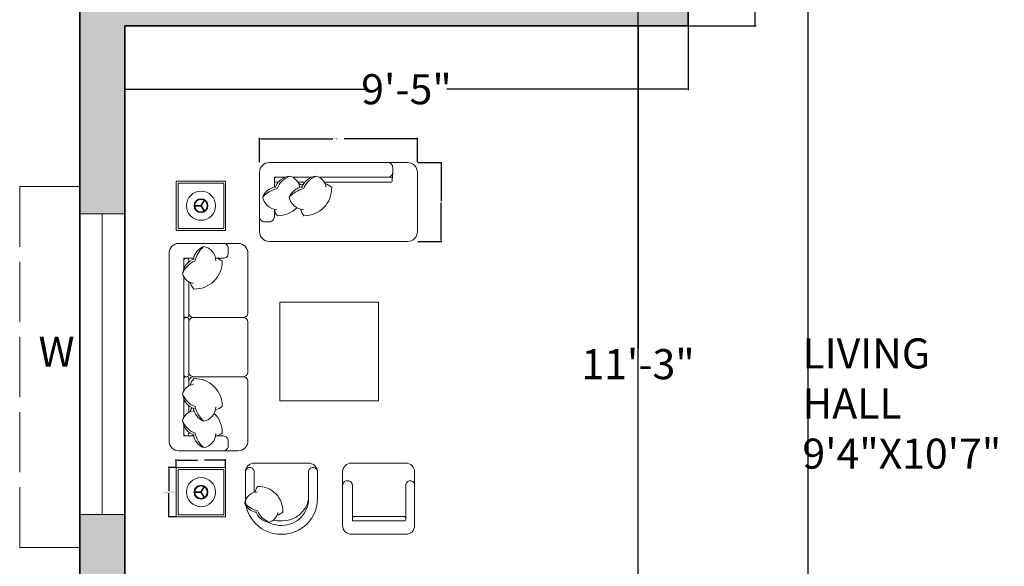
# Model space of a CAD drawing. Units: inches. Extents: x -5 to 482, y -460 to 66.
# Tile 13 of 31: x 21 to 218, y -252 to -143. Entities that reach past the tile are written whole.
import ezdxf

# ---------------------------------------------------------------- set-up
doc = ezdxf.new("R2010")
doc.units = ezdxf.units.IN
doc.header["$MEASUREMENT"] = 0
doc.linetypes.add('ACAD_ISO02W100', pattern=[15, 12, -3])
for name, color, linetype, lineweight in [('A-ANNO-DIMS', 2, 'Continuous', 18), ('A-ANNO-TEXT', 7, 'Continuous', 18), ('A-AREA-IDEN', 7, 'Continuous', 18), ('A-FURN', 8, 'Continuous', 18), ('A-GLAZ', 4, 'Continuous', 18), ('A-GLAZ-OVHD', 4, 'ACAD_ISO02W100', 13), ('A-WALL', 7, 'Continuous', 35), ('A-WALL-PATT', 152, 'Continuous', 13)]:
    doc.layers.add(name, color=color, linetype=linetype, lineweight=lineweight)
doc.styles.get("Standard").update_dxf_attribs({"font": 'arial.ttf'})
doc.dimstyles.get("Standard").update_dxf_attribs({"dimtxt": 0.18, "dimasz": 0.18, "dimexe": 0.18, "dimexo": 0.0625, "dimgap": 0.09, "dimtad": 0, "dimtih": 1, "dimtoh": 1, "dimdec": 0, "dimzin": 0, "dimdsep": 46, "dimlunit": 3, "dimtxsty": 'Standard', "dimcen": 0.09, "dimadec": 0, "dimazin": 0, "dimtfac": 1, "dimtdec": 0, "dimtofl": 0, "dimtmove": 0, "dimatfit": 3, "dimfxl": 1, "dimtolj": 1, "dimtzin": 0, "dimarcsym": 0})

# ---------------------------------------------------------------- blocks, each defined once
blk = doc.blocks.new('DAY BED1')
at = {"color": 0}
blk.add_line((0.3, 0.25), (0.225, 0.2549), dxfattribs=at)
blk.add_lwpolyline([(-0.3, 0, -0.414214), (-0.4, 0.1), (-0.4, 0.1, 0.317837), (-0.4, 0.1, -0.414214), (-0.4, 0.1), (-0.4, 0.1, 1.186185), (-0.4, 0.1, -0.414214), (-0.4, 0.1), (-0.4, 1.5, -0.414214), (-0.3, 1.6), (0.3, 1.6, -0.414214), (0.4, 1.5), (0.4, 0.1, -0.414214), (0.3, 0)], format="xyb", close=True, dxfattribs=at)
for points in [[(-0.0725, 1.45), (-0.15, 1.45, -0.414214), (-0.2, 1.5), (-0.2, 1.55, -0.414214), (-0.15, 1.6)], [(-0.0756, 1.4249, -0.356772), (0.0505, 1.5682, -0.249542), (0.1543, 1.4384, 9.61688)], [(0.0505, 1.5682, -0.14773), (0.1364, 1.422, -0.213343), (0.2624, 1.2931, -0.178662)], [(-0.0725, 1.4501, 0.165541), (-0.1386, 1.4192, 0.200231), (-0.0581, 1.2207, 0.121523)], [(0.1433, 1.4422, -0.306663), (0.2624, 1.2931, -0.30633), (0.1536, 1.1957, 0.872847)], [(0.25, 1.3448), (0.25, 1.45), (0.1517, 1.45, -0.414214)], [(0.2, 1.4118), (0.2, 1.43, -0.414214), (0.22, 1.45), (0.23, 1.45, -0.414214), (0.25, 1.43)], [(0.25, 1.43), (0.25, 1.3448, -0.414214)], [(-0.0756, 1.1556, -0.356772), (0.0505, 1.2988, -0.249542), (0.1543, 1.169, 9.61688)], [(0.0505, 1.2988, -0.14773), (0.1364, 1.1527, -0.213343), (0.2624, 1.0238, -0.178662)], [(0.1678, 1.1631, 0.071865), (0.1873, 1.205, -7.115464)], [(0.2, 1.1425), (0.2, 1.2113, -0.414214)], [(0.25, 1.2616), (0.25, 1.0755, -0.414214)], [(-0.0725, 1.1808, 0.165541), (-0.1386, 1.1498, 0.425989), (0.1479, 0.869, 0.121523), (0.1873, 0.9357, -7.115464)], [(0.1433, 1.1729, -0.306663), (0.2624, 1.0238, -0.30633), (0.1536, 0.9263, 0.872847)], [(0.25, 0.9923), (0.25, 0.2749, -0.414214), (0.23, 0.2549), (0.22, 0.2549, -0.414214), (0.2, 0.2749), (0.2, 0.9419, -0.414214)], [(0.25, 0.3775), (0.25, 0.3, 0.414214), (0.3, 0.25), (0.35, 0.25, 0.414214), (0.4, 0.3)]]:
    blk.add_lwpolyline(points, format="xyb", dxfattribs=at)
for points in [[(0.25, 1.0755), (0.25, 1.2616)], [(0.25, 0.3775), (0.25, 0.9923)]]:
    blk.add_lwpolyline(points, dxfattribs=at)
blk = doc.blocks.new('*D8')
at = {"layer": 'A-ANNO-DIMS', "color": 0, "lineweight": -2, "transparency": 16777216}
for p, q in [((154.44, 4.15), (167.95, 4.15)), ((167.77, 3.97), (167.77, -66.95)), ((167.77, -144.17), (167.77, -73.25)), ((154.44, -144.35), (167.95, -144.35))]:
    blk.add_line(p, q, dxfattribs=at)
at = {"layer": 'A-ANNO-DIMS', "color": 0, "transparency": 16777216}
for points in [[(167.74, 3.97), (167.8, 3.97), (167.77, 4.15)], [(167.74, -144.17), (167.8, -144.17), (167.77, -144.35)]]:
    blk.add_solid(points, dxfattribs=at)
at = {"layer": 'Defpoints', "color": 0, "transparency": 16777216}
for p in [(154.38, 4.15), (167.77, 4.15), (154.38, -144.35)]:
    blk.add_point(p, dxfattribs=at)
at = {"layer": 'A-ANNO-DIMS', "color": 0, "transparency": 16777216, "insert": (167.77, -70.1), "char_height": 6, "attachment_point": 5}
blk.add_mtext('\\A1;12\'-5"', dxfattribs=at)
blk = doc.blocks.new('*D18')
at = {"layer": 'A-ANNO-DIMS', "color": 0, "lineweight": -2, "transparency": 16777216}
for p, q in [((144.38, -144.53), (144.38, -208.69)), ((144.44, -144.35), (144.56, -144.35)), ((144.38, -279.17), (144.38, -215)), ((144.44, -279.35), (144.56, -279.35))]:
    blk.add_line(p, q, dxfattribs=at)
at = {"layer": 'A-ANNO-DIMS', "color": 0, "transparency": 16777216}
for points in [[(144.35, -144.53), (144.41, -144.53), (144.38, -144.35)], [(144.35, -279.17), (144.41, -279.17), (144.38, -279.35)]]:
    blk.add_solid(points, dxfattribs=at)
at = {"layer": 'Defpoints', "color": 0, "transparency": 16777216}
for p in [(144.38, -144.35), (144.38, -144.35), (144.38, -279.35)]:
    blk.add_point(p, dxfattribs=at)
at = {"layer": 'A-ANNO-DIMS', "color": 0, "transparency": 16777216, "insert": (144.38, -211.85), "char_height": 6, "attachment_point": 5}
blk.add_mtext('\\A1;11\'-3"', dxfattribs=at)
blk = doc.blocks.new('*D19')
at = {"layer": 'A-ANNO-DIMS', "color": 0, "lineweight": -2, "transparency": 16777216}
for p, q in [((41.88, -144.41), (41.88, -157.16)), ((154.38, -144.41), (154.38, -157.16)), ((42.06, -156.98), (90.06, -156.98)), ((154.2, -156.98), (106.19, -156.98))]:
    blk.add_line(p, q, dxfattribs=at)
at = {"layer": 'A-ANNO-DIMS', "color": 0, "transparency": 16777216}
for points in [[(42.06, -156.95), (42.06, -157.01), (41.88, -156.98)], [(154.2, -156.95), (154.2, -157.01), (154.38, -156.98)]]:
    blk.add_solid(points, dxfattribs=at)
at = {"layer": 'Defpoints', "color": 0, "transparency": 16777216}
for p in [(41.88, -144.35), (154.38, -144.35), (41.88, -156.98)]:
    blk.add_point(p, dxfattribs=at)
at = {"layer": 'A-ANNO-DIMS', "color": 0, "transparency": 16777216, "insert": (98.13, -156.98), "char_height": 6, "attachment_point": 5}
blk.add_mtext('\\A1;9\'-5"', dxfattribs=at)
blk = doc.blocks.new('WIN-GLAZ-60IN')
for p, q in [((0, 9), (60, 9)), ((0, 4.5), (60, 4.5)), ((60, 0), (0, 0))]:
    blk.add_line(p, q)
blk = doc.blocks.new('WIN-SHADE-72IN')
for p, q in [((0, 12), (72, 12)), ((0, 12), (0, 0)), ((72, 12), (72, 0))]:
    blk.add_line(p, q)
blk = doc.blocks.new('END-TABLE-WITH-LAMP')
for p, q in [((4.87, 4.96), (5.57, 6.16)), ((4.98, 4.9), (5.68, 6.1)), ((4.93, 4.99), (3.54, 4.99)), ((4.93, 4.86), (3.54, 4.86)), ((4.87, 4.9), (5.57, 3.69)), ((4.98, 4.96), (5.68, 3.75))]:
    blk.add_line(p, q)
at = {"ltscale": 0.03}
blk.add_lwpolyline([(9.85, 9.85), (9.85, 0), (0, 0), (0, 9.85)], close=True, dxfattribs=at)
blk.add_lwpolyline([(9.46, 0.39), (9.46, 9.46), (0.39, 9.46), (0.39, 0.39)], close=True)
for radius in [2.91, 1.39, 1.25]:
    blk.add_circle((4.93, 4.93), radius)
blk = doc.blocks.new('*D53')
at = {"layer": 'A-ANNO-DIMS', "color": 0, "lineweight": -2, "transparency": 16777216}
for p, q in [((52.1, -232.46), (50.5, -232.46)), ((50.68, -232.64), (50.68, -237.2)), ((50.68, -242.13), (50.68, -237.56)), ((52.1, -242.31), (50.5, -242.31))]:
    blk.add_line(p, q, dxfattribs=at)
at = {"layer": 'A-ANNO-DIMS', "color": 0, "transparency": 16777216}
for points in [[(50.65, -232.64), (50.71, -232.64), (50.68, -232.46)], [(50.65, -242.13), (50.71, -242.13), (50.68, -242.31)]]:
    blk.add_solid(points, dxfattribs=at)
at = {"layer": 'Defpoints', "color": 0, "transparency": 16777216}
for p in [(50.68, -232.46), (52.16, -232.46), (52.16, -242.31)]:
    blk.add_point(p, dxfattribs=at)
at = {"layer": 'A-ANNO-DIMS', "color": 0, "transparency": 16777216, "insert": (50.68, -237.38), "char_height": 0.18, "attachment_point": 5}
blk.add_mtext('\\A1;END TABLE 0\'-10" TYP.', dxfattribs=at)
blk = doc.blocks.new('*D54')
at = {"layer": 'A-ANNO-DIMS', "color": 0, "lineweight": -2, "transparency": 16777216}
for p, q in [((52.16, -232.39), (52.16, -230.8)), ((52.34, -230.98), (56.38, -230.98)), ((61.83, -230.98), (57.79, -230.98)), ((62.01, -232.39), (62.01, -230.8))]:
    blk.add_line(p, q, dxfattribs=at)
at = {"layer": 'A-ANNO-DIMS', "color": 0, "transparency": 16777216}
for points in [[(52.34, -230.95), (52.34, -231.01), (52.16, -230.98)], [(61.83, -230.95), (61.83, -231.01), (62.01, -230.98)]]:
    blk.add_solid(points, dxfattribs=at)
at = {"layer": 'Defpoints', "color": 0, "transparency": 16777216}
for p in [(62.01, -230.98), (52.16, -232.46), (62.01, -232.46)]:
    blk.add_point(p, dxfattribs=at)
at = {"layer": 'A-ANNO-DIMS', "color": 0, "transparency": 16777216, "insert": (57.09, -230.98), "char_height": 0.18, "attachment_point": 5}
blk.add_mtext('\\A1;0\'-10" TYP.', dxfattribs=at)
blk = doc.blocks.new('*D65')
at = {"layer": 'A-ANNO-DIMS', "color": 0, "lineweight": -2, "transparency": 16777216}
for p, q in [((68.78, -171.55), (68.78, -166.7)), ((68.96, -166.88), (83.42, -166.88)), ((100.13, -166.88), (85.66, -166.88)), ((100.31, -171.55), (100.31, -166.7))]:
    blk.add_line(p, q, dxfattribs=at)
at = {"layer": 'A-ANNO-DIMS', "color": 0, "transparency": 16777216}
for points in [[(68.96, -166.85), (68.96, -166.91), (68.78, -166.88)], [(100.13, -166.85), (100.13, -166.91), (100.31, -166.88)]]:
    blk.add_solid(points, dxfattribs=at)
at = {"layer": 'Defpoints', "color": 0, "transparency": 16777216}
for p in [(68.78, -166.88), (68.78, -171.61), (100.31, -171.61)]:
    blk.add_point(p, dxfattribs=at)
at = {"layer": 'A-ANNO-DIMS', "color": 0, "transparency": 16777216, "insert": (84.54, -166.88), "char_height": 0.18, "attachment_point": 5}
blk.add_mtext('\\A1;DAY BED 2\'-7 1/2"', dxfattribs=at)
blk = doc.blocks.new('*D66')
at = {"layer": 'A-ANNO-DIMS', "color": 0, "lineweight": -2, "transparency": 16777216}
for p, q in [((100.37, -171.61), (105.22, -171.61)), ((105.04, -171.79), (105.04, -179.31)), ((105.04, -187.19), (105.04, -179.67)), ((100.37, -187.37), (105.22, -187.37))]:
    blk.add_line(p, q, dxfattribs=at)
at = {"layer": 'A-ANNO-DIMS', "color": 0, "transparency": 16777216}
for points in [[(105.01, -171.79), (105.07, -171.79), (105.04, -171.61)], [(105.01, -187.19), (105.07, -187.19), (105.04, -187.37)]]:
    blk.add_solid(points, dxfattribs=at)
at = {"layer": 'Defpoints', "color": 0, "transparency": 16777216}
for p in [(100.31, -171.61), (105.04, -171.61), (100.31, -187.37)]:
    blk.add_point(p, dxfattribs=at)
at = {"layer": 'A-ANNO-DIMS', "color": 0, "transparency": 16777216, "insert": (105.04, -179.49), "char_height": 0.18, "attachment_point": 5}
blk.add_mtext('\\A1;1\'-4"', dxfattribs=at)
blk = doc.blocks.new('*D73')
at = {"layer": 'A-ANNO-DIMS', "color": 0, "lineweight": -2, "transparency": 16777216}
for p, q in [((144.38, -295.8), (144.38, 50.93)), ((144.56, 50.75), (160.98, 50.75)), ((178.2, 50.75), (161.78, 50.75)), ((178.38, -295.8), (178.38, 50.93))]:
    blk.add_line(p, q, dxfattribs=at)
at = {"layer": 'A-ANNO-DIMS', "color": 0, "transparency": 16777216}
for points in [[(144.56, 50.78), (144.56, 50.72), (144.38, 50.75)], [(178.2, 50.78), (178.2, 50.72), (178.38, 50.75)]]:
    blk.add_solid(points, dxfattribs=at)
at = {"layer": 'Defpoints', "color": 0, "transparency": 16777216}
for p in [(178.38, 50.75), (144.38, -295.86), (178.38, -295.86)]:
    blk.add_point(p, dxfattribs=at)
at = {"layer": 'A-ANNO-DIMS', "color": 0, "transparency": 16777216, "insert": (161.38, 50.75), "char_height": 0.18, "attachment_point": 5}
blk.add_mtext('\\A1;2\'-10"', dxfattribs=at)

msp = doc.modelspace()

# ---------------------------------------------------------------- hatches: boundary and pattern name
at = {"layer": 'A-WALL-PATT'}
h = msp.add_hatch(color=256, dxfattribs=at)
h.dxf.hatch_style = 1
h.paths.add_polyline_path([(149.38, -412.85), (144.38, -412.85), (144.38, -283.85), (144.38, -279.35), (133.88, -279.35), (133.88, -283.85), (139.88, -283.85), (139.88, -412.85), (133.51, -412.85), (133.51, -413.92), (102.65, -413.92), (102.65, -421.02), (133.51, -421.02), (133.51, -421.85), (149.38, -421.85)])
h.paths.add_polyline_path([(226.05, -412.85), (218.88, -412.85), (218.88, -350.85), (262.88, -350.85), (262.88, -386.85), (267.38, -386.85), (267.38, -283.85), (270.38, -283.85), (270.38, -279.35), (244.88, -279.35), (244.88, -283.85), (262.88, -283.85), (262.88, -346.35), (218.88, -346.35), (218.88, -283.85), (220.88, -283.85), (220.88, -279.35), (214.38, -279.35), (214.38, -283.85), (214.38, -412.85), (209.38, -412.85), (209.38, -421.85), (226.05, -421.85)])
h.paths.add_polyline_path([(315.81, -412.85), (250.05, -412.85), (250.05, -421.85), (315.81, -421.85)])
h.paths.add_polyline_path([(430.38, -378.35), (421.38, -378.35), (421.38, -412.85), (375.81, -412.85), (375.81, -421.85), (430.38, -421.85)])
h.paths.add_polyline_path([(78.69, -413.92), (47.68, -413.92), (47.68, -412.85), (41.88, -412.85), (41.88, -283.85), (109.88, -283.85), (109.88, -279.35), (41.88, -279.35), (41.88, -241.85), (32.88, -241.85), (32.88, -421.85), (47.68, -421.85), (47.68, -421.02), (78.69, -421.02)])
h.paths.add_polyline_path([(41.88, -144.35), (154.38, -144.35), (154.38, -137.85), (149.88, -137.85), (149.88, -139.85), (41.88, -139.85), (41.88, -97.85), (32.88, -97.85), (32.88, -181.85), (41.88, -181.85)])
h.paths.add_polyline_path([(430.38, -241.85), (421.38, -241.85), (421.38, -279.35), (309.38, -279.35), (309.38, -170.35), (304.88, -170.35), (304.88, -279.35), (294.38, -279.35), (294.38, -283.85), (421.38, -283.85), (421.38, -318.35), (430.38, -318.35)])
h.paths.add_polyline_path([(430.38, -119.85), (421.38, -119.85), (421.38, -139.85), (419.38, -139.85), (419.38, -144.35), (421.38, -144.35), (421.38, -181.85), (430.38, -181.85)])
h.paths.add_polyline_path([(395.38, -139.85), (377.38, -139.85), (377.38, -75.85), (421.38, -75.85), (421.38, -95.85), (430.38, -95.85), (430.38, -45.6), (421.38, -45.6), (421.38, -71.35), (377.38, -71.35), (377.38, -22.85), (372.88, -22.85), (372.88, -139.85), (242.88, -139.85), (242.88, -137.85), (238.38, -137.85), (238.38, -144.35), (304.88, -144.35), (304.88, -146.35), (309.38, -146.35), (309.38, -144.35), (395.38, -144.35)])
h.paths.add_polyline_path([(65.88, 13.15), (32.88, 13.15), (32.88, -37.85), (41.88, -37.85), (41.88, 4.15), (65.88, 4.15)])
h.paths.add_polyline_path([(166.38, 13.15), (125.88, 13.15), (125.88, 4.15), (149.88, 4.15), (149.88, -113.85), (154.38, -113.85), (154.38, 4.15), (166.38, 4.15)])
h.paths.add_polyline_path([(277.88, 13.15), (226.38, 13.15), (226.38, 4.15), (238.38, 4.15), (238.38, -113.85), (242.88, -113.85), (242.88, 4.15), (277.88, 4.15)])
h.paths.add_polyline_path([(430.38, 13.15), (337.88, 13.15), (337.88, 4.15), (372.88, 4.15), (372.88, 1.15), (377.38, 1.15), (377.38, 4.15), (421.38, 4.15), (421.38, -21.6), (430.38, -21.6)])

# ---------------------------------------------------------------- linework, layer by layer
at = {"layer": 'A-FURN', "ltscale": 0.03}
for points in [[(64.5, -187.75, -0.414214), (66.47, -189.72), (66.47, -201.54, -0.414214), (65.49, -202.53, -0.414214), (66.47, -203.51), (66.47, -213.37, -0.414214), (65.49, -214.35, -0.414214), (66.47, -215.34), (66.47, -227.16, -0.414214), (64.5, -229.13), (52.68, -229.13, -0.414214), (50.71, -227.16), (50.71, -189.72, -0.414214), (52.68, -187.75)], [(97.98, -245.8), (97.98, -245.8, 0.414214), (99.76, -244.03), (99.76, -233.37, 0.414214), (97.98, -231.59), (97.98, -231.59), (87.14, -231.59, 0.414214), (85.37, -233.37), (85.37, -244.03, 0.414214), (87.14, -245.8)]]:
    msp.add_lwpolyline(points, format="xyb", close=True, dxfattribs=at)
at = {"layer": 'A-FURN'}
for points in [[(57.6, -188.37, 0.14773), (55.9, -191.25, 0.213343), (53.42, -193.8, 0.178662)], [(60.08, -191.2, 0.356772), (57.6, -188.37, 0.249542), (55.55, -190.93, -9.61688)], [(61.55, -187.75, -0.414214), (62.53, -188.73), (62.53, -189.72, -0.414214), (61.55, -190.7), (60.02, -190.7)], [(54.65, -191.46), (54.65, -191.1, 0.414214), (54.26, -190.7), (54.06, -190.7, 0.414214), (53.66, -191.1)], [(60.02, -190.7, -0.165541), (61.32, -191.31, -0.425989), (55.68, -196.85, -0.121523), (54.9, -195.53, 7.115464)], [(55.77, -190.86, 0.306663), (53.42, -193.8, 0.30633), (55.56, -195.72, -0.872847)], [(53.66, -191.1), (53.66, -192.78, 0.414214)], [(53.66, -194.42), (53.66, -202.13, 0.414214), (54.06, -202.53), (54.26, -202.53, 0.414214), (54.65, -202.13), (54.65, -195.41, 0.414214)], [(54.65, -201.54, 0.414214), (55.63, -202.53), (65.49, -202.53, 0.414214)], [(54.65, -203.51, -0.414214), (55.63, -202.53)], [(54.65, -213.37, 0.414214), (55.63, -214.35)], [(55.77, -220.72, -0.306663), (53.42, -217.78, -0.30633), (55.56, -215.86, 0.872847)], [(53.66, -217.16), (53.66, -214.75, -0.414214), (54.06, -214.35), (54.26, -214.35, -0.414214), (54.65, -214.75), (54.65, -216.16, -0.414214)], [(54.65, -215.34, -0.414214), (55.63, -214.35), (65.49, -214.35, -0.414214)], [(60.02, -220.87, 0.165541), (61.32, -220.26, 0.425989), (55.68, -214.73, 0.121523), (54.9, -216.04, -7.115464)], [(57.6, -223.2, -0.14773), (55.9, -220.32, -0.213343), (53.42, -217.78, -0.178662)], [(53.66, -222.46), (53.66, -218.8, -0.414214)], [(54.65, -220.12), (54.65, -221.47, -0.414214)], [(55.77, -226.02, -0.306663), (53.42, -223.08, -0.30633), (55.56, -221.16, 0.872847)], [(55.28, -220.52, 0.071865), (54.9, -221.35, -7.115464)], [(60.08, -220.37, -0.356772), (57.6, -223.2, -0.249542), (55.55, -220.64, 9.61688)], [(60.02, -226.18, 0.165541), (61.32, -225.57, 0.200231), (59.74, -221.66, 0.121523)], [(57.6, -228.51, -0.14773), (55.9, -225.63, -0.213343), (53.42, -223.08, -0.178662)], [(53.66, -224.1), (53.66, -226.18), (55.6, -226.18, -0.414214)], [(53.66, -225.78), (53.66, -224.1, -0.414214)], [(54.65, -225.42), (54.65, -225.78, -0.414214), (54.26, -226.18), (54.06, -226.18, -0.414214), (53.66, -225.78)], [(60.08, -225.68, -0.356772), (57.6, -228.51, -0.249542), (55.55, -225.95, 9.61688)], [(60.02, -226.18), (61.55, -226.18, -0.414214), (62.53, -227.16), (62.53, -228.15, -0.414214), (61.55, -229.13)], [(67.73, -237.45), (67.73, -233.37, 0.414214), (66.84, -232.48), (66.84, -232.48, 0.414214), (65.95, -233.37)], [(78.57, -238.7), (78.57, -233.37, -0.414214), (79.45, -232.48), (79.45, -232.48, -0.414214), (80.34, -233.37)], [(85.37, -236.03, -0.414214), (86.25, -235.14), (86.43, -235.14, -0.414214), (87.32, -236.03), (87.32, -237.41)], [(97.98, -242.61), (97.98, -236.03, -0.414214), (98.87, -235.14), (98.87, -235.14, -0.414214), (99.76, -236.03)], [(68.35, -237.35, 0.356772), (65.81, -239.59, 0.249542), (68.11, -241.44, -9.61688)], [(67.9, -237.41, -0.165541), (68.45, -236.23, -0.425989), (73.44, -241.32, -0.121523), (72.26, -242.03, 7.115464)], [(65.81, -239.59, 0.14773), (68.4, -241.12, 0.213343), (70.69, -243.36, 0.178662)], [(78.57, -238.7, -0.372719), (73.24, -243.14), (73.15, -243.14)], [(78.57, -238.7, -0.414214), (73.24, -244.03), (73.15, -244.03)], [(68.04, -241.24, 0.306663), (70.69, -243.36, 0.30633), (72.42, -241.43, -0.872847)], [(70.41, -243.32, 0.130591), (73.06, -244.03), (73.15, -244.03)], [(71.54, -242.95, 0.072384), (73.06, -243.14), (73.15, -243.14)], [(91.56, -242.25), (87.68, -242.25, 0.414214), (87.32, -242.61), (87.32, -242.78, 0.414214), (87.68, -243.14)], [(87.68, -243.14), (90.67, -243.14, 0.414214)], [(90.67, -243.14), (97.63, -243.14, 0.414214), (97.98, -242.78), (97.98, -242.61, 0.414214), (97.63, -242.25), (91.56, -242.25, 0.414214)]]:
    msp.add_lwpolyline(points, format="xyb", dxfattribs=at)
for points in [[(55.6, -190.7), (53.66, -190.7), (53.66, -192.78)], [(53.66, -194.42), (53.66, -217.16)], [(53.66, -218.8), (53.66, -222.46)], [(87.32, -237.41), (87.32, -243.14), (90.67, -243.14)], [(90.67, -243.14), (97.89, -243.14)]]:
    msp.add_lwpolyline(points, dxfattribs=at)
at = {"layer": 'A-FURN', "ltscale": 0.03}
msp.add_lwpolyline([(92.56, -219.15), (92.56, -199.45), (72.85, -199.45), (72.85, -219.15)], close=True, dxfattribs=at)
at = {"layer": 'A-FURN'}
msp.add_lwpolyline([(53.66, -213.96), (53.66, -202.92, -0.414214), (54.06, -202.53), (54.26, -202.53, -0.414214), (54.65, -202.92), (54.65, -213.96, -0.414214), (54.26, -214.35), (54.06, -214.35, -0.414214)], format="xyb", close=True, dxfattribs=at)
at = {"layer": 'A-FURN', "ltscale": 0.03}
msp.add_lwpolyline([(73.15, -231.59), (78.57, -231.59, -0.414214), (80.34, -233.37), (80.34, -238.7, -0.414214), (73.24, -245.8), (73.15, -245.8), (73.06, -245.8, -0.414214), (65.95, -238.7), (65.95, -233.37, -0.414214), (67.73, -231.59), (73.15, -231.59)], format="xyb", dxfattribs=at)
at = {"layer": 'A-GLAZ'}
for p, q in [((41.88, -181.85), (32.88, -181.85)), ((32.88, -241.85), (41.88, -241.85))]:
    msp.add_line(p, q, dxfattribs=at)
at = {"layer": 'A-WALL'}
for p, q in [((32.88, 13.15), (32.88, -421.85)), ((154.38, -137.85), (154.38, -144.35)), ((41.88, -144.35), (154.38, -144.35)), ((41.88, -144.35), (41.88, -279.35))]:
    msp.add_line(p, q, dxfattribs=at)

# ---------------------------------------------------------------- block references
at = {"layer": 'A-FURN', "ltscale": 0.03, "xscale": 19.70694952145727, "yscale": 19.70694952145727, "zscale": 19.70694952145727, "rotation": 90}
msp.add_blockref('DAY BED1', (100.31, -179.49), dxfattribs=at)
at = {"layer": 'A-FURN'}
for p in [(52.16, -185.16), (52.16, -242.31)]:
    msp.add_blockref('END-TABLE-WITH-LAMP', p, dxfattribs=at)
at = {"layer": 'A-GLAZ', "rotation": 90.00000000000003}
msp.add_blockref('WIN-GLAZ-60IN', (41.88, -241.85), dxfattribs=at)
at = {"layer": 'A-GLAZ-OVHD', "rotation": 90}
msp.add_blockref('WIN-SHADE-72IN', (32.88, -248.41), dxfattribs=at)

# ---------------------------------------------------------------- texts
at = {"layer": 'A-ANNO-TEXT', "insert": (24.64, -206.37), "char_height": 6, "attachment_point": 1}
msp.add_mtext('W', dxfattribs=at)
at = {"layer": 'A-AREA-IDEN', "insert": (177.2, -206.7), "char_height": 6, "attachment_point": 1}
msp.add_mtext_dynamic_manual_height_columns('LIVING HALL\\P9\'4"X10\'7"', width=8.2666, gutter_width=1, heights=[0], dxfattribs=at)

# ---------------------------------------------------------------- dimensions: what is measured, and where the dimension line sits
at = {"layer": 'A-ANNO-DIMS'}
for base, p1, p2, override, picture, middle in [((178.38, 50.75), (144.38, -295.86), (178.38, -295.86), {"dimdec": 1, "dimlfac": 1, "dimrnd": 0, "dimzin": 1, "dimdsep": 46, "dimlunit": 4, "dimfrac": 2}, '*D73', (161.38, 50.75)), ((41.87673599, -156.98412235), (154.37673599, -144.34866403), (41.87673599, -144.34866403), {"dimtxt": 6, "dimclrd": 0, "dimclre": 0, "dimclrt": 0}, '*D19', (98.12673599, -156.98412235))]:
    dim = msp.add_linear_dim(base=base, p1=p1, p2=p2, dimstyle='Standard', override=override, dxfattribs=at)
    dim.commit()
    dim.dimension.update_dxf_attribs({"geometry": picture, "text_midpoint": middle})
for base, p1, p2, override, picture, middle in [((167.76833102, 4.15133597), (154.37673599, -144.34866403), (154.37673599, 4.15133597), {"dimtxt": 6, "dimclrd": 0, "dimclre": 0, "dimclrt": 0}, '*D8', (167.76833102, -70.09866403)), ((144.38, -144.35), (144.38, -279.35), (144.38, -144.35), {"dimtxt": 6, "dimclrd": 0, "dimclre": 0, "dimclrt": 0}, '*D18', (144.38, -211.85)), ((105.04, -171.61), (100.31, -187.37), (100.31, -171.61), {"dimdec": 1, "dimlfac": 1, "dimrnd": 0, "dimzin": 1, "dimdsep": 46, "dimlunit": 4, "dimfrac": 2}, '*D66', (105.04, -179.49))]:
    dim = msp.add_linear_dim(base=base, p1=p1, p2=p2, angle=90, dimstyle='Standard', override=override, dxfattribs=at)
    dim.commit()
    dim.dimension.update_dxf_attribs({"geometry": picture, "text_midpoint": middle})
for base, p1, p2, angle, text, picture, middle in [((68.78, -166.88), (100.31, -171.61), (68.78, -171.61), 180, 'DAY BED <>', '*D65', (84.54, -166.88)), ((50.6811, -232.4557), (52.1591, -242.3091), (52.1591, -232.4557), 90, 'END TABLE <> TYP.', '*D53', (50.6811, -237.3824))]:
    dim = msp.add_linear_dim(base=base, p1=p1, p2=p2, angle=angle, text=text, dimstyle='Standard', override={"dimdec": 1, "dimlfac": 1, "dimrnd": 0, "dimzin": 1, "dimdsep": 46, "dimlunit": 4, "dimfrac": 2}, dxfattribs=at)
    dim.commit()
    dim.dimension.update_dxf_attribs({"geometry": picture, "text_midpoint": middle})
dim = msp.add_linear_dim(base=(62.0126, -230.9776), p1=(52.1591, -232.4557), p2=(62.0126, -232.4557), text='<> TYP.', dimstyle='Standard', override={"dimdec": 1, "dimlfac": 1, "dimrnd": 0, "dimzin": 1, "dimdsep": 46, "dimlunit": 4, "dimfrac": 2}, dxfattribs=at)
dim.commit()
dim.dimension.update_dxf_attribs({"geometry": '*D54', "text_midpoint": (57.0858, -230.9776)})

doc.saveas('drawing.dxf')
